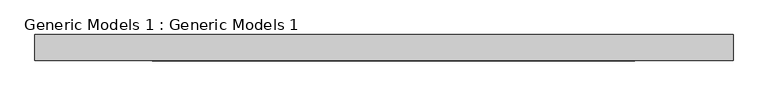
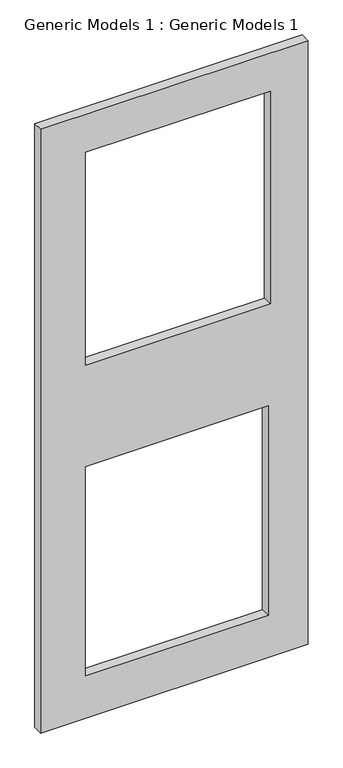
"""IFC4 building model written with IfcOpenShell, lengths in millimetres: proxy geometry, Generic Models 1 : Generic Models 1."""

from ifc_helpers import new_model, si_unit, frame, origin, place, context, project, spatial, polyline, outline, extrude, source, transform, mapped, element, save


def generic_models_1_generic_models_1_954afae2(model_context):
    return source(origin(), model_context, "Body", "SweptSolid", [
        extrude(outline(polyline([(6934.2, -7687.479089), (6934.2, -10408.429089), (446.4, -10408.429089), (446.4, -7687.479089), (6934.2, -7687.479089)]), holes=[polyline([(6525.0, -8071.629089), (4239.0, -8071.629089), (4239.0, -9951.229089), (6525.0, -9951.229089), (6525.0, -8071.629089)]), polyline([(3150.0, -8090.3545103), (900.0, -8090.3545103), (900.0, -9951.229089), (3150.0, -9951.229089), (3150.0, -8090.3545103)])]), frame((0.0, -4695.4968048, 0.0), z_axis=(0.0, 1.0, 0.0), x_axis=(0.0, 0.0, 1.0)), (0.0, 0.0, 1.0), 101.6),
    ])


if __name__ == "__main__":
    model = new_model("IFC4")
    model_context = context("Model", 3, world=origin())
    ifc_project = project(units=[si_unit("LENGTHUNIT", "METRE", prefix="MILLI")], contexts=[model_context])
    site = spatial("IfcSite", under=ifc_project)
    building = spatial("IfcBuilding", under=site)
    placement = place(None, origin())
    generic_models_1_generic_models_1_shape = generic_models_1_generic_models_1_954afae2(model_context)
    element("IfcBuildingElementProxy", 1, Name="Generic Models 1 : Generic Models 1", ObjectType="Generic Models 1 : Generic Models 1", at=placement, inside=building, context=model_context, shape_type="MappedRepresentation", body=[
        mapped(generic_models_1_generic_models_1_shape, transform((0.0, 0.0, 0.0), x_axis=(1.0, 0.0, 0.0), y_axis=(0.0, 1.0, 0.0), z_axis=(0.0, 0.0, 1.0))),
    ])
    save(model, "model.ifc")
